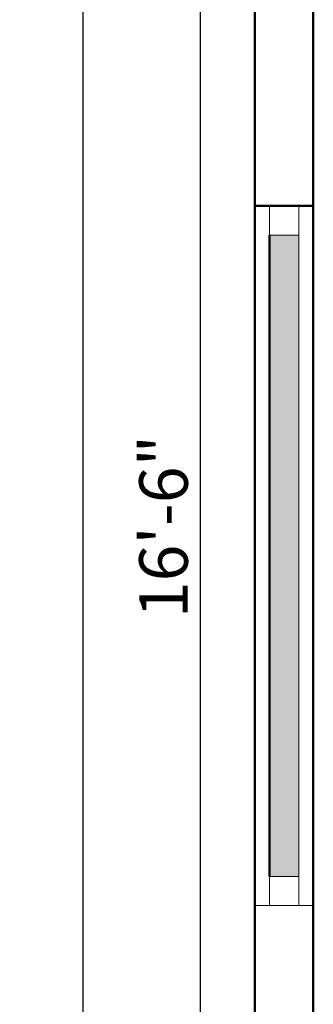
# Model space of a CAD drawing. Units: inches. Extents: x 3064 to 19385, y 846 to 15425.
# Tile 67 of 108: x 6445 to 6475, y 1624 to 1725. Entities that reach past the tile are written whole.
import ezdxf

# ---------------------------------------------------------------- set-up
doc = ezdxf.new("R2010")
doc.units = ezdxf.units.IN
for name, color, linetype, lineweight in [('A-ANNO-DIMS', 2, 'Continuous', 18), ('A-GLAZ', 4, 'Continuous', 18), ('A-WALL', 7, 'Continuous', 50)]:
    doc.layers.add(name, color=color, linetype=linetype, lineweight=lineweight)
doc.styles.get("Standard").update_dxf_attribs({"font": 'arial.ttf'})
doc.dimstyles.new('ISO-25', dxfattribs={"dimtxt": 9, "dimasz": 2.5, "dimexe": 1.25, "dimexo": 0.625, "dimtad": 1, "dimdec": 1, "dimlunit": 3, "dimtxsty": 'Standard', "dimcen": 2.5, "dimadec": 0, "dimazin": 0, "dimtfac": 1, "dimtdec": 1, "dimtmove": 0, "dimatfit": 3, "dimfxl": 1, "dimarcsym": 0})

# ---------------------------------------------------------------- blocks, each defined once
blk = doc.blocks.new('*D372')
at = {"layer": 'A-ANNO-DIMS', "color": 0, "lineweight": -2, "transparency": 16777216}
for p, q in [((6474.41, 1771.99), (6462.18, 1771.99)), ((6463.43, 1576.49), (6463.43, 1769.49)), ((6474.41, 1573.99), (6462.18, 1573.99))]:
    blk.add_line(p, q, dxfattribs=at)
at = {"layer": 'A-ANNO-DIMS', "color": 0, "transparency": 16777216}
for points in [[(6463.02, 1769.49), (6463.85, 1769.49), (6463.43, 1771.99)], [(6463.02, 1576.49), (6463.85, 1576.49), (6463.43, 1573.99)]]:
    blk.add_solid(points, dxfattribs=at)
at = {"layer": 'Defpoints', "color": 0, "transparency": 16777216}
for p in [(6463.43, 1771.99), (6475.03, 1771.99), (6475.03, 1573.99)]:
    blk.add_point(p, dxfattribs=at)
at = {"layer": 'A-ANNO-DIMS', "color": 0, "transparency": 16777216, "insert": (6460.26, 1672.99), "char_height": 5, "attachment_point": 5, "rotation": 90}
blk.add_mtext('16\'-6"', dxfattribs=at)
blk = doc.blocks.new('*D370')
at = {"layer": 'A-ANNO-DIMS', "color": 0, "lineweight": -2, "transparency": 16777216}
for p, q in [((6468.41, 1987.99), (6450.1, 1987.99)), ((6451.35, 1498.49), (6451.35, 1985.49)), ((6468.41, 1495.99), (6450.1, 1495.99))]:
    blk.add_line(p, q, dxfattribs=at)
at = {"layer": 'A-ANNO-DIMS', "color": 0, "transparency": 16777216}
for points in [[(6450.94, 1985.49), (6451.77, 1985.49), (6451.35, 1987.99)], [(6450.94, 1498.49), (6451.77, 1498.49), (6451.35, 1495.99)]]:
    blk.add_solid(points, dxfattribs=at)
at = {"layer": 'Defpoints', "color": 0, "transparency": 16777216}
for p in [(6451.35, 1987.99), (6469.03, 1987.99), (6469.03, 1495.99)]:
    blk.add_point(p, dxfattribs=at)
at = {"layer": 'A-ANNO-DIMS', "color": 0, "transparency": 16777216, "insert": (6448.22, 1741.99), "char_height": 5, "attachment_point": 5, "rotation": 90}
blk.add_mtext("41'", dxfattribs=at)
blk = doc.blocks.new('WIN-1900')
blk.add_line((3, 0), (3, 66))
blk.add_lwpolyline([(3, 66), (0, 66), (0, 69), (3, 69)], close=True)

msp = doc.modelspace()

# ---------------------------------------------------------------- hatches: boundary and pattern name
at = {"layer": 'A-GLAZ'}
h = msp.add_hatch(color=256, dxfattribs=at)
h.dxf.hatch_style = 1
h.paths.add_polyline_path([(6470.53, 1636.99), (6473.53, 1636.99), (6473.53, 1702.99), (6470.53, 1702.99)])

# ---------------------------------------------------------------- linework, layer by layer
msp.add_line((6475.03, 1633.99), (6469.03, 1633.99), dxfattribs=at)
msp.add_lwpolyline([(6473.53, 1633.99), (6470.53, 1633.99), (6470.53, 1636.99), (6473.53, 1636.99)], close=True, dxfattribs=at)
at = {"layer": 'A-WALL'}
for p, q in [((6469.03, 1987.99), (6469.03, 1567.99)), ((6475.03, 1771.99), (6475.03, 1573.99)), ((6475.03, 1705.99), (6469.03, 1705.99)), ((6470.53, 1636.99), (6470.53, 1702.99))]:
    msp.add_line(p, q, dxfattribs=at)

# ---------------------------------------------------------------- block references
at = {"layer": 'A-GLAZ'}
msp.add_blockref('WIN-1900', (6470.53, 1636.99), dxfattribs=at)

# ---------------------------------------------------------------- dimensions: what is measured, and where the dimension line sits
at = {"layer": 'A-ANNO-DIMS'}
for base, p1, p2, override, picture, middle in [((6451.35, 1987.99), (6469.03, 1495.99), (6469.03, 1987.99), {"dimtxt": 5, "dimclrd": 0, "dimclre": 0, "dimclrt": 0}, '*D370', (6448.22, 1741.99)), ((6463.43, 1771.99), (6475.03, 1573.99), (6475.03, 1771.99), {"dimtxt": 5, "dimclrd": 0, "dimclre": 0, "dimclrt": 0, "dimtmove": 1}, '*D372', (6460.26, 1672.99))]:
    dim = msp.add_linear_dim(base=base, p1=p1, p2=p2, angle=90, dimstyle='ISO-25', override=override, dxfattribs=at)
    dim.commit()
    dim.dimension.update_dxf_attribs({"geometry": picture, "text_midpoint": middle})

doc.saveas('drawing.dxf')
